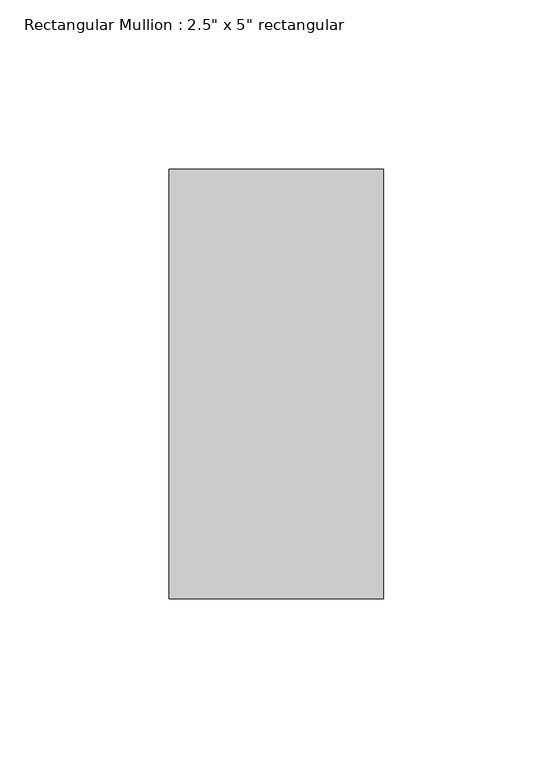
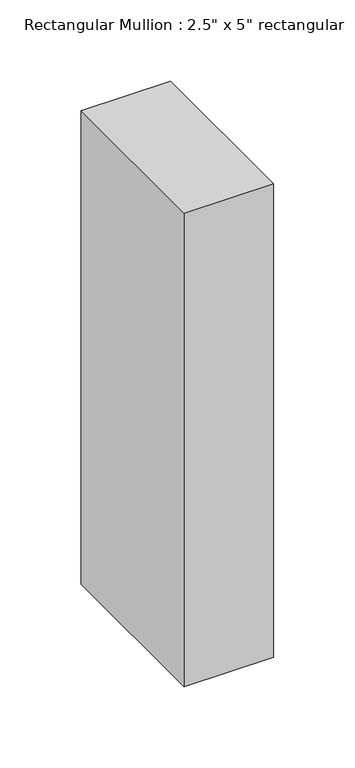
"""IFC4 building model written with IfcOpenShell, lengths in millimetres: member geometry."""

from ifc_helpers import new_model, si_unit, frame, origin, place, context, project, spatial, polyline, outline, extrude, source, transform, mapped, element, save


def member_ca359333(model_context):
    return source(origin(), model_context, "Body", "SweptSolid", [
        extrude(outline(polyline([(31.75, 63.5), (31.75, -63.5), (-31.75, -63.5), (-31.75, 63.5), (31.75, 63.5)])), frame((0.0, 0.0, -355.6), z_axis=(0.0, 0.0, 1.0), x_axis=(1.0, 0.0, 0.0)), (0.0, 0.0, 1.0), 355.6),
    ])


if __name__ == "__main__":
    model = new_model("IFC4")
    model_context = context("Model", 3, world=origin())
    ifc_project = project(units=[si_unit("LENGTHUNIT", "METRE", prefix="MILLI")], contexts=[model_context])
    site = spatial("IfcSite", under=ifc_project)
    building = spatial("IfcBuilding", under=site)
    placement = place(None, origin())
    member_shape = member_ca359333(model_context)
    element("IfcMember", 1, ObjectType="Rectangular Mullion : 2.5\" x 5\" rectangular", at=placement, inside=building, context=model_context, shape_type="MappedRepresentation", body=[
        mapped(member_shape, transform((0.0, 0.0, 0.0), x_axis=(1.0, 0.0, 0.0), y_axis=(0.0, 1.0, 0.0), z_axis=(0.0, 0.0, 1.0))),
    ])
    save(model, "model.ifc")

# Revit data of these elements
# Type "Rectangular Mullion : 2.5\" x 5\" rectangular"
#   built-in parameter 1007304 = 0.416667 (stored number, unit not read)
#   built-in parameter 1007301 = 0.104167 (stored number, unit not read)
#   built-in parameter 1007300 = 0.104167 (stored number, unit not read)
